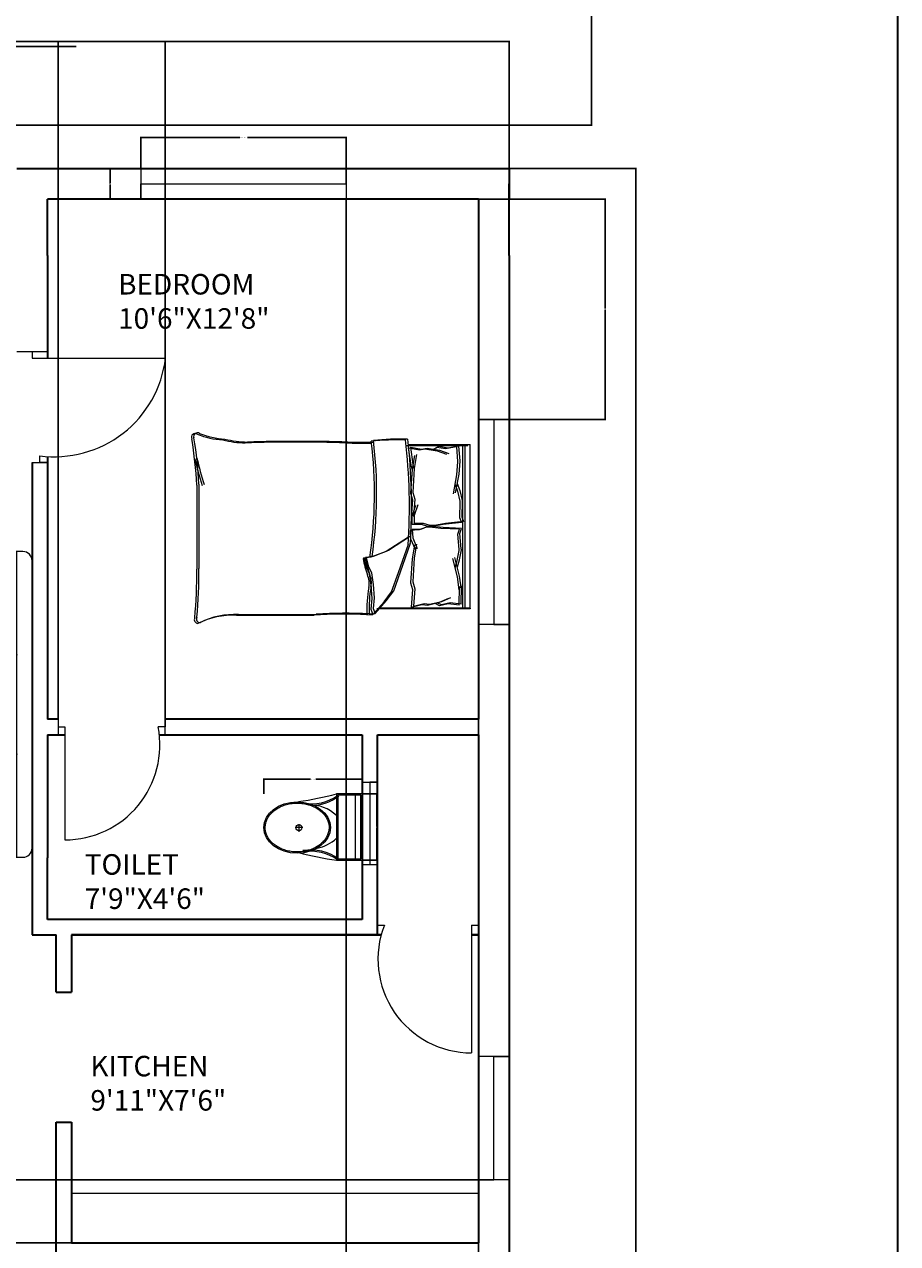
# Model space of a CAD drawing. Units: inches. Extents: x 1854 to 2495, y 1460 to 2772.
# Tile 11 of 12: x 2239 to 2495, y 1958 to 2314. Entities that reach past the tile are written whole.
import ezdxf

# ---------------------------------------------------------------- set-up
doc = ezdxf.new("R2010")
doc.units = ezdxf.units.IN
for name, color, linetype, lineweight in [('A-ANNO-DIMS', 2, 'Continuous', 18), ('A-ANNO-TEXT', 7, 'Continuous', 25), ('A-ANNO-TTLB', 7, 'Continuous', 35), ('A-AREA-IDEN', 7, 'Continuous', 18), ('A-DOOR', 3, 'Continuous', 18), ('A-FLOR-CASE', 8, 'Continuous', 18), ('A-FLOR-FIXT', 9, 'Continuous', 18), ('A-FURN', 8, 'Continuous', 13), ('A-GLAZ', 4, 'Continuous', 18), ('A-WALL', 7, 'Continuous', 35)]:
    doc.layers.add(name, color=color, linetype=linetype, lineweight=lineweight)
doc.styles.get("Standard").update_dxf_attribs({"font": 'arial.ttf'})
doc.dimstyles.get("Standard").update_dxf_attribs({"dimtxt": 0.18, "dimasz": 0.18, "dimexe": 0.18, "dimexo": 0.0625, "dimgap": 0.09, "dimtad": 0, "dimtih": 1, "dimtoh": 1, "dimdec": 4, "dimzin": 0, "dimdsep": 46, "dimtxsty": 'Standard', "dimcen": 0.09, "dimadec": 0, "dimazin": 0, "dimtfac": 1, "dimtdec": 4, "dimtofl": 0, "dimtmove": 0, "dimatfit": 3, "dimfxl": 1, "dimtolj": 1, "dimtzin": 0, "dimarcsym": 0})

# ---------------------------------------------------------------- blocks, each defined once
blk = doc.blocks.new('A$C31115884')
for p, q in [((283.1, 497.7), (223.4, 497.7)), ((257.5, 466.4), (257.5, 523.2)), ((0, 200), (0, 0)), ((520, 200), (0, 200)), ((520, 0), (520, 200)), ((10, 190), (10, 10)), ((510, 190), (10, 190)), ((510, 10), (510, 190)), ((510, 54.5), (0, 54.5)), ((10, 10), (510, 10)), ((0, 0), (520, 0))]:
    blk.add_line(p, q)
blk.add_circle((255.6, 496.4), 23.6)
for centre, radius, start, end in [((2777.7, -204.6), 2807, 165.4549, 171.71327), ((3237, 905), 2807, 188.28673, 194.5451), ((-294.5, 403.3), 364.7, 324.20913, 9.34987), ((-294.5, 403.3), 374.7, 324.20913, 9.34987), ((139.5, 406.2), 293.5, 315.84364, 2.65635), ((805.8, 403.3), 374.7, 179.20365, 215.79087), ((805.8, 403.3), 364.7, 170.65013, 215.79087), ((383.6, 406.2), 293.5, 190.27735, 224.15636)]:
    blk.add_arc(centre, radius, start, end)
blk.add_ellipse((256.2, 509.9), major_axis=(0, -260.7), ratio=0.772727)
blk.add_open_spline([(256.2, 259.2), (263.1, 259.2), (270, 259.7), (287.8, 262.3), (298.7, 265.1), (319.9, 273.1), (330.2, 278.4), (350.1, 291.1), (359.7, 298.7), (377.7, 315.9), (386.2, 325.5), (401.7, 346.6), (408.8, 358.1), (421.3, 382.5), (426.8, 395.5), (435.9, 422.4), (439.5, 436.4), (444.8, 465.1), (446.5, 479.7), (447.9, 509.2), (447.6, 524), (445, 553.3), (442.7, 567.8), (436.3, 596), (432.1, 609.7), (421.9, 636), (416, 648.6), (402.5, 672.1), (395, 683), (378.6, 703), (369.8, 712.1), (351.1, 728), (341.3, 734.8), (320.9, 746.2), (310.4, 750.7), (288.9, 757.3), (278, 759.4), (256, 761), (245, 760.6), (223.1, 757.2), (212.3, 754.3), (191.1, 746.1), (180.8, 740.7), (160.9, 727.8), (151.4, 720.1), (133.5, 702.7), (125.1, 693), (109.6, 671.7), (102.6, 660.2), (90.2, 635.7), (84.9, 622.7), (76, 595.6), (72.4, 581.6), (67.2, 552.9), (65.6, 538.2), (64.4, 508.8), (64.8, 494), (67.5, 464.7), (69.9, 450.2), (76.6, 422), (80.8, 408.3), (91.1, 382.2), (97.2, 369.7), (110.8, 346.3), (118.4, 335.4), (134.8, 315.6), (143.7, 306.7), (162.4, 290.9), (172.3, 284.2), (192.8, 273), (203.3, 268.6), (224.8, 262.2), (235.8, 260.2), (249.9, 259.3), (253, 259.2), (256.2, 259.2)], degree=3, knots=[0, 0, 0, 0, 0.110105, 0.110105, 0.285049, 0.285049, 0.459994, 0.459994, 0.634938, 0.634938, 0.809882, 0.809882, 0.984827, 0.984827, 1.159771, 1.159771, 1.334715, 1.334715, 1.50966, 1.50966, 1.684604, 1.684604, 1.859549, 1.859549, 2.034493, 2.034493, 2.209437, 2.209437, 2.384382, 2.384382, 2.559326, 2.559326, 2.73427, 2.73427, 2.909215, 2.909215, 3.084159, 3.084159, 3.259103, 3.259103, 3.434048, 3.434048, 3.608992, 3.608992, 3.783936, 3.783936, 3.958881, 3.958881, 4.133825, 4.133825, 4.30877, 4.30877, 4.483714, 4.483714, 4.658658, 4.658658, 4.833603, 4.833603, 5.008547, 5.008547, 5.183491, 5.183491, 5.358436, 5.358436, 5.53338, 5.53338, 5.708324, 5.708324, 5.883269, 5.883269, 6.058213, 6.058213, 6.233158, 6.233158, 6.283185, 6.283185, 6.283185, 6.283185])
blk = doc.blocks.new('BED-DOUBLE')
for p, q in [((0, 51.27), (0, 51.49)), ((0, 51.49), (0.64, 51.49)), ((0, 51.27), (26.61, 51.27)), ((0, 51.27), (26.61, 51.27)), ((0, 51.27), (0, 3.48)), ((0.64, 51.49), (27.25, 51.49)), ((0.64, 51.49), (27.25, 51.49)), ((1.53, 3.48), (1.53, 51.27)), ((1.53, 3.48), (1.53, 51.27)), ((2.17, 3.7), (2.17, 51.49)), ((2.17, 3.7), (2.17, 51.49)), ((2.56, 50.11), (2.46, 44.71)), ((2.56, 50.11), (2.46, 44.71)), ((2.56, 50.11), (5.77, 49.73)), ((2.56, 50.11), (5.77, 49.73)), ((3.2, 50.34), (3.1, 44.94)), ((3.2, 50.34), (3.1, 44.94)), ((3.2, 50.34), (6.41, 49.96)), ((3.2, 50.34), (6.41, 49.96)), ((5.77, 49.73), (8.34, 50.33)), ((5.77, 49.73), (8.34, 50.33)), ((6.41, 49.96), (8.98, 50.56)), ((6.41, 49.96), (8.98, 50.56)), ((11.83, 50.11), (8.26, 49.31)), ((11.83, 50.11), (8.26, 49.31)), ((8.34, 50.33), (9.38, 49.81)), ((8.34, 50.33), (9.38, 49.81)), ((12.47, 50.34), (8.9, 49.54)), ((12.47, 50.34), (8.9, 49.54)), ((8.98, 50.56), (10.02, 50.04)), ((8.98, 50.56), (10.02, 50.04)), ((13.43, 49.92), (11.83, 50.11)), ((13.43, 49.92), (11.83, 50.11)), ((14.07, 50.15), (12.47, 50.34)), ((14.07, 50.15), (12.47, 50.34)), ((16.57, 50.7), (13.43, 49.92)), ((16.57, 50.7), (13.43, 49.92)), ((17.21, 50.93), (14.07, 50.15)), ((17.21, 50.93), (14.07, 50.15)), ((16.17, 45.57), (16.57, 50.7)), ((16.17, 45.57), (16.57, 50.7)), ((16.81, 45.8), (17.21, 50.93)), ((16.81, 45.79), (17.21, 50.93)), ((27.75, 52.87), (24.5, 49.16)), ((27.75, 52.87), (24.5, 49.16)), ((28.39, 53.1), (25.14, 49.39)), ((28.39, 53.1), (25.14, 49.39)), ((29.49, 52.95), (27.75, 52.87, 3.87)), ((29.49, 52.95), (27.75, 52.87, 3.87)), ((28.37, 51.33), (27.75, 52.87)), ((28.37, 51.33), (27.75, 52.87)), ((28.06, 48.23), (28.37, 51.33)), ((28.06, 48.23), (28.37, 51.33)), ((30.13, 53.18), (28.39, 53.1, 3.87)), ((30.13, 53.18), (28.39, 53.1, 3.87)), ((29, 51.56), (28.39, 53.1)), ((29, 51.56), (28.39, 53.1)), ((28.7, 48.46), (29, 51.56)), ((28.7, 48.46), (29, 51.56)), ((8.26, 49.31), (5.58, 48.13)), ((8.26, 49.31), (5.58, 48.13)), ((8.9, 49.54), (6.22, 48.36)), ((8.9, 49.54), (6.22, 48.36)), ((22.97, 46.45), (20.96, 40.87)), ((22.97, 46.45), (20.96, 40.87)), ((24.5, 49.16), (22.33, 46.22)), ((24.5, 49.16), (22.33, 46.22)), ((25.14, 49.39), (22.97, 46.45)), ((25.14, 49.39), (22.97, 46.45)), ((28.37, 44.36), (28.06, 48.23)), ((28.37, 44.36), (28.06, 48.23)), ((29, 44.59), (28.7, 48.46)), ((29, 44.59), (28.7, 48.46)), ((2.46, 44.71), (2.54, 45.71)), ((2.46, 44.71), (2.54, 45.71)), ((2.54, 45.71), (3.07, 41.91)), ((2.54, 45.71), (3.07, 41.91)), ((3.1, 44.94), (3.18, 45.94)), ((3.1, 44.94), (3.18, 45.94)), ((3.18, 45.94), (3.71, 42.14)), ((3.18, 45.94), (3.71, 42.14)), ((16.73, 43.61), (16.17, 45.57)), ((16.73, 43.61), (16.17, 45.57)), ((16.3, 36.6), (16.73, 43.61)), ((16.3, 36.6), (16.73, 43.61)), ((17.37, 43.83), (16.81, 45.8)), ((17.37, 43.83), (16.81, 45.79)), ((16.93, 36.82), (17.37, 43.83)), ((16.93, 36.82), (17.37, 43.83)), ((22.33, 46.22), (20.32, 40.64)), ((22.33, 46.22), (20.32, 40.64)), ((28.83, 40.95), (28.37, 44.36)), ((28.83, 40.95), (28.37, 44.36)), ((29.47, 41.18), (29, 44.59)), ((29.47, 41.18), (29, 44.59)), ((3.07, 41.91), (4.42, 36.5)), ((3.07, 41.91), (4.42, 36.5)), ((3.67, 39.2), (3.08, 37.14)), ((3.67, 39.2), (3.08, 37.14)), ((3.71, 42.14), (5.06, 36.72)), ((3.71, 42.14), (5.06, 36.72)), ((4.31, 39.43), (3.72, 37.36)), ((4.31, 39.43), (3.72, 37.36)), ((20.32, 40.64), (17.38, 32.31)), ((20.32, 40.64), (17.38, 32.31)), ((20.96, 40.87), (18.02, 32.53)), ((20.96, 40.87), (18.02, 32.53)), ((29.76, 38.94), (28.83, 40.95)), ((29.76, 38.94), (28.83, 40.95)), ((30.4, 39.17), (29.47, 41.18)), ((30.4, 39.17), (29.47, 41.18)), ((79.25, 15.06), (79.25, 39.68)), ((79.25, 15.06), (79.25, 39.68)), ((79.88, 15.29), (79.88, 39.91)), ((79.88, 15.29), (79.88, 39.91)), ((3.08, 37.14), (2.54, 34.2)), ((3.08, 37.14), (2.54, 34.2)), ((3.72, 37.36), (3.18, 34.43)), ((3.72, 37.36), (3.18, 34.43)), ((15.63, 32.56), (16.3, 36.6)), ((15.63, 32.56), (16.3, 36.6)), ((16.27, 32.79), (16.93, 36.82)), ((16.27, 32.79), (16.93, 36.82)), ((23.88, 34.45), (28.37, 36.15)), ((23.88, 34.45), (28.37, 36.15)), ((24.52, 34.68), (29, 36.38)), ((24.52, 34.68), (29, 36.38)), ((28.37, 36.15), (30.38, 36.46)), ((28.37, 36.15), (30.38, 36.46)), ((29, 36.38), (31.02, 36.69)), ((29, 36.38), (31.02, 36.69)), ((30.38, 36.46), (29.76, 38.94)), ((30.38, 36.46), (29.76, 38.94)), ((31.02, 36.69), (30.4, 39.17)), ((31.02, 36.69), (30.4, 39.17)), ((2.54, 34.2), (2.56, 33.88)), ((2.54, 34.2), (2.56, 33.88)), ((2.56, 33.88), (2.98, 29.46)), ((2.56, 33.88), (2.98, 29.46)), ((3.18, 34.43), (3.2, 34.11)), ((3.18, 34.43), (3.2, 34.11)), ((3.2, 34.11), (3.62, 29.68)), ((3.2, 34.11), (3.62, 29.68)), ((16.74, 30.75), (15.45, 33.82)), ((16.74, 30.75), (15.45, 33.82)), ((17.38, 30.98), (16.09, 34.05)), ((17.38, 30.98), (16.09, 34.05)), ((17.38, 30.26), (23.88, 34.45)), ((17.38, 30.26), (23.88, 34.45)), ((18.02, 30.49), (24.52, 34.68)), ((18.02, 30.49), (24.52, 34.68)), ((2.98, 29.46), (2.49, 27.98)), ((2.98, 29.46), (2.49, 27.98)), ((3.62, 29.68), (3.13, 28.21)), ((3.62, 29.68), (3.13, 28.21)), ((14.86, 28.36), (17.53, 28.53)), ((14.86, 28.36), (17.53, 28.53)), ((16.89, 28.3), (16.74, 30.75)), ((16.89, 28.3), (16.74, 30.75)), ((17.53, 28.53), (17.38, 30.98)), ((17.53, 28.53), (17.38, 30.98)), ((1.87, 25.98), (7.22, 26.56)), ((1.87, 25.98), (7.22, 26.56)), ((2.45, 24.54), (1.87, 25.98)), ((2.45, 24.54), (1.87, 25.98)), ((2.49, 27.98), (7.87, 27.73)), ((2.49, 27.98), (7.87, 27.73)), ((2.51, 26.21), (7.86, 26.79)), ((2.51, 26.21), (7.86, 26.79)), ((3.09, 24.77), (2.51, 26.21)), ((3.09, 24.77), (2.51, 26.21)), ((3.13, 28.21), (8.51, 27.96)), ((3.13, 28.21), (8.51, 27.96)), ((7.22, 26.56), (10.4, 27.14)), ((7.22, 26.56), (10.4, 27.14)), ((7.86, 26.79), (11.04, 27.37)), ((7.86, 26.79), (11.04, 27.37)), ((7.87, 27.73), (11.08, 27.36)), ((7.87, 27.73), (11.08, 27.35)), ((8.51, 27.96), (11.72, 27.58)), ((8.51, 27.96), (11.72, 27.58)), ((10.4, 27.14), (11.7, 27.14)), ((10.4, 27.14), (11.7, 27.14)), ((11.04, 27.37), (12.34, 27.37)), ((11.04, 27.37), (12.34, 27.37)), ((11.08, 27.36), (12.38, 27.44)), ((11.08, 27.35), (12.38, 27.44)), ((11.7, 27.14), (13.58, 26.56)), ((11.7, 27.14), (13.58, 26.56)), ((11.72, 27.58), (13.02, 27.66)), ((11.72, 27.58), (13.02, 27.66)), ((12.34, 27.37), (14.22, 26.79)), ((12.34, 27.37), (14.22, 26.79)), ((12.38, 27.44), (14.22, 28.13)), ((12.38, 27.44), (14.22, 28.13)), ((13.02, 27.66), (14.86, 28.36)), ((13.02, 27.66), (14.86, 28.36)), ((13.58, 26.56), (16.26, 26.56)), ((13.58, 26.56), (16.26, 26.56)), ((14.22, 28.13), (16.89, 28.3)), ((14.22, 28.13), (16.89, 28.3)), ((14.22, 26.79), (16.9, 26.79)), ((14.22, 26.79), (16.9, 26.79)), ((16.26, 26.56), (16.26, 24.1)), ((16.26, 26.56), (16.26, 24.1)), ((16.9, 26.79), (16.9, 24.33)), ((16.9, 26.79), (16.9, 24.33)), ((2.3, 20.09), (2.45, 24.54)), ((2.3, 20.09), (2.45, 24.54)), ((2.94, 20.32), (3.09, 24.77)), ((2.94, 20.32), (3.09, 24.77)), ((16.26, 24.1), (15.17, 20.96)), ((16.26, 24.1), (15.17, 20.96)), ((16.9, 24.33), (15.81, 21.19)), ((16.9, 24.33), (15.81, 21.19)), ((16.17, 19.38), (16.57, 24.52)), ((16.17, 19.38), (16.57, 24.52)), ((16.81, 19.61), (17.21, 24.74)), ((16.81, 19.61), (17.21, 24.74)), ((2.3, 19.77), (2.3, 20.09)), ((2.3, 19.77), (2.3, 20.09)), ((3.03, 16.88), (2.3, 19.77)), ((3.03, 16.88), (2.3, 19.77)), ((2.94, 20), (2.94, 20.32)), ((2.94, 20), (2.94, 20.32)), ((3.67, 17.11), (2.94, 20)), ((3.67, 17.11), (2.94, 20)), ((3.96, 12.34), (4.97, 17.83)), ((3.96, 12.34), (4.97, 17.83)), ((16.73, 17.42), (16.17, 19.38)), ((16.73, 17.42), (16.17, 19.38)), ((17.37, 17.65), (16.81, 19.61)), ((17.37, 17.65), (16.81, 19.61)), ((3.75, 14.86), (3.03, 16.88)), ((3.75, 14.85), (3.03, 16.88)), ((3.32, 12.11), (4.33, 17.6)), ((3.32, 12.11), (4.33, 17.6)), ((4.39, 15.08), (3.67, 17.11)), ((4.39, 15.08), (3.67, 17.11)), ((16.3, 10.41), (16.73, 17.42)), ((16.3, 10.41), (16.73, 17.42)), ((16.93, 10.64), (17.37, 17.65)), ((16.93, 10.64), (17.37, 17.65)), ((3.03, 8.29), (3.32, 12.11)), ((3.03, 8.28), (3.32, 12.11)), ((3.67, 8.51), (3.96, 12.34)), ((3.67, 8.51), (3.96, 12.34)), ((3.01, 8.18), (3.03, 8.29)), ((3.01, 8.18), (3.03, 8.28)), ((3.34, 3.9), (3.01, 8.18)), ((3.34, 3.9), (3.01, 8.18)), ((3.65, 8.41), (3.67, 8.51)), ((3.65, 8.41), (3.67, 8.51)), ((3.98, 4.13), (3.65, 8.41)), ((3.98, 4.13), (3.65, 8.41)), ((15.63, 6.38), (16.3, 10.41)), ((15.63, 6.38), (16.3, 10.41)), ((16.27, 6.61), (16.93, 10.64)), ((16.27, 6.61), (16.93, 10.64)), ((16.3, 10.41), (16.62, 9.28)), ((16.3, 10.41), (16.62, 9.28)), ((16.62, 9.28), (17.34, 4.18)), ((16.62, 9.28), (17.34, 4.18)), ((16.93, 10.64), (17.26, 9.51)), ((16.93, 10.64), (17.26, 9.51)), ((17.26, 9.51), (17.98, 4.41)), ((17.26, 9.51), (17.98, 4.41)), ((18.75, 3.7), (0.64, 3.7)), ((18.75, 3.7), (0.64, 3.7)), ((3.32, 3.89), (6.5, 4.47)), ((3.32, 3.89), (6.5, 4.47)), ((3.96, 4.12), (7.14, 4.7)), ((3.96, 4.12), (7.14, 4.7)), ((8.96, 5.05), (6.21, 6.06)), ((8.96, 5.05), (6.21, 6.06)), ((6.5, 4.47), (9.1, 4.04)), ((6.5, 4.47), (9.1, 4.04)), ((9.59, 5.28), (6.85, 6.29)), ((9.59, 5.28), (6.85, 6.29)), ((7.14, 4.7), (9.74, 4.27)), ((7.14, 4.7), (9.74, 4.27)), ((12.57, 4.47), (8.96, 5.05)), ((12.57, 4.47), (8.96, 5.05)), ((9.1, 4.04), (10.11, 4.62)), ((9.1, 4.04), (10.11, 4.62)), ((13.21, 4.7), (9.59, 5.28)), ((13.21, 4.7), (9.59, 5.28)), ((9.74, 4.27), (10.75, 4.85)), ((9.74, 4.27), (10.75, 4.85)), ((14.16, 4.76), (12.57, 4.47)), ((14.16, 4.76), (12.57, 4.47)), ((14.8, 4.99), (13.21, 4.7)), ((14.8, 4.99), (13.21, 4.7)), ((17.34, 4.18), (14.16, 4.76)), ((17.34, 4.18), (14.16, 4.76)), ((17.98, 4.41), (14.8, 4.99)), ((17.98, 4.41), (14.8, 4.99)), ((18.11, 3.48), (0, 3.48)), ((18.11, 3.48), (0, 3.48))]:
    blk.add_line(p, q)
for centre, radius, start, end in [((68.67, 76.16), 23.07, 267.4714, 296.4681), ((68.67, 76.16), 23.07, 267.4714, 296.4681), ((69.31, 76.39), 23.07, 267.4714, 296.4681), ((69.31, 76.39), 23.07, 267.4714, 296.4681), ((78.87, 54.41), 1.1, 332.6588, 86.02), ((78.87, 54.41), 1.1, 332.6588, 86.02), ((212.28, 41.15), 133.04, 174.4998, 180.6351), ((212.28, 41.15), 133.04, 174.4998, 180.6351), ((79.51, 54.64), 1.1, 332.6588, 86.02), ((79.51, 54.64), 1.1, 332.6588, 86.02), ((212.92, 41.38), 133.04, 174.4998, 180.6351), ((212.92, 41.38), 133.04, 174.4998, 180.6351), ((-6.66, 51.33), 36.18, 349.8763, 2.5657), ((-6.66, 51.33), 36.18, 349.8763, 2.5657), ((36.32, 182.27), 129.5, 266.9791, 273.8365), ((36.32, 182.27), 129.5, 266.9791, 273.8365), ((-6.02, 51.56), 36.18, 349.8763, 2.5657), ((-6.02, 51.56), 36.18, 349.8763, 2.5657), ((36.95, 182.49), 129.5, 266.9791, 273.8365), ((36.95, 182.49), 129.5, 266.9791, 273.8365), ((67.82, -4508.74), 4561.86, 90.00217, 90.28689), ((67.82, -4508.74), 4561.86, 90.00217, 90.28689), ((68.46, -4508.51), 4561.86, 90.00217, 90.28689), ((68.46, -4508.52), 4561.86, 90.00217, 90.28689), ((35.07, 43.74), 6.22, 168.6608, 203.7384), ((35.07, 43.74), 6.22, 168.6608, 203.7384), ((35.71, 43.97), 6.22, 168.6608, 203.7384), ((35.71, 43.97), 6.22, 168.6608, 203.7384), ((1.48, 31.15), 29.65, 10.6617, 19.8806), ((1.48, 31.15), 29.65, 10.6617, 19.8806), ((2.12, 31.38), 29.65, 10.6617, 19.8806), ((2.12, 31.38), 29.65, 10.6617, 19.8806), ((156.32, 17.76), 129.02, 171.7845, 186.9006), ((156.32, 17.76), 129.02, 171.7845, 186.9006), ((156.96, 17.98), 129.02, 171.7845, 186.9006), ((156.96, 17.98), 129.02, 171.7845, 186.9006), ((30.44, 36.64), 0.185, 250.2464, 1.1377), ((30.44, 36.64), 0.185, 250.2464, 1.1377), ((31.08, 36.86), 0.185, 250.2464, 1.1377), ((31.08, 36.86), 0.185, 250.2464, 1.1377), ((182.05, 21.36), 164.97, 176.0865, 186.7821), ((182.05, 21.36), 164.97, 176.0865, 186.7821), ((182.69, 21.59), 164.97, 176.0865, 186.7821), ((182.69, 21.59), 164.97, 176.0865, 186.7821), ((-23.71, -17.22), 106.46, 13.3832, 17.7053), ((-23.71, -17.22), 106.46, 13.3832, 17.7053), ((-23.07, -16.99), 106.46, 13.3832, 17.7053), ((-23.07, -16.99), 106.46, 13.3832, 17.7053), ((200.84, 21.43), 121.76, 182.9958, 189.4091), ((200.84, 21.43), 121.76, 182.9958, 189.4091), ((201.48, 21.66), 121.76, 182.9958, 189.4091), ((201.48, 21.66), 121.76, 182.9958, 189.4091), ((20.1, 85.16), 83.31, 268.7218, 275.604), ((20.1, 85.16), 83.31, 268.7218, 275.604), ((20.74, 85.39), 83.31, 268.7218, 275.604), ((20.74, 85.39), 83.31, 268.7218, 275.604), ((31.17, -167.31), 170.11, 88.4762, 91.0082), ((31.17, -167.31), 170.11, 88.4762, 91.0082), ((31.81, -167.08), 170.11, 88.4762, 91.0082), ((31.81, -167.08), 170.11, 88.4762, 91.0082), ((50.61, 484.82), 482.31, 268.2277, 271.7185), ((50.61, 484.82), 482.31, 268.2277, 271.7185), ((51.25, 485.05), 482.31, 268.2277, 271.7185), ((51.25, 485.05), 482.31, 268.2277, 271.7185), ((64.52, -26.9), 29.63, 76.0648, 88.9113), ((64.52, -26.9), 29.63, 76.0648, 88.9113), ((65.15, -26.67), 29.63, 76.0648, 88.9113), ((65.15, -26.67), 29.63, 76.0648, 88.9113), ((70.28, -21.66), 23.56, 67.9751, 86.652), ((70.28, -21.66), 23.56, 67.9751, 86.652), ((70.92, -21.43), 23.56, 67.9751, 86.652), ((70.92, -21.43), 23.56, 67.9751, 86.652), ((79.72, 1.09), 1.09, 236.1736, 23.4781), ((79.72, 1.09), 1.09, 236.1736, 23.4781), ((80.36, 1.32), 1.09, 236.1736, 23.4781), ((80.36, 1.32), 1.09, 236.1736, 23.4781)]:
    blk.add_arc(centre, radius, start, end)
blk = doc.blocks.new('WINDOW-60IN')
for p, q in [((0, 9), (0, 0)), ((60, 4.5), (60, 9)), ((60, 9), (60, 0)), ((0, 0), (0, 4.5)), ((0, 4.5), (60, 4.5))]:
    blk.add_line(p, q)
blk = doc.blocks.new('WINDOW-36IN')
for p, q in [((0, 36), (9, 36)), ((9, 36), (4.5, 36)), ((4.5, 36), (4.5, 0)), ((4.5, 0), (0, 0)), ((0, 0), (9, 0))]:
    blk.add_line(p, q)
blk = doc.blocks.new('WINDOW-VENT-24IN-INTERIOR')
for p, q in [((0, 24), (4.5, 24)), ((2.25, 24), (2.25, 0)), ((0, 0), (4.5, 0))]:
    blk.add_line(p, q)
blk = doc.blocks.new('SOFA-3-SEAT')
for points in [[(2.23, 59.19), (21.22, 59.19, 0.414214), (23.45, 61.43), (23.45, 87.12, 0.414214), (21.22, 89.35), (2.23, 89.35, 0.414214), (0, 87.12), (0, 61.43, 0.414214)], [(2.23, 59.19), (21.22, 59.19, -0.414214), (23.45, 56.96), (23.45, 32.39, -0.414214), (21.22, 30.16), (2.23, 30.16, -0.414214), (0, 32.39), (0, 56.96, -0.414214)], [(2.23, 0), (21.22, 0, 0.414214), (23.45, 2.23), (23.45, 27.92, 0.414214), (21.22, 30.16), (2.23, 30.16, 0.414214), (0, 27.92), (0, 2.23, 0.414214)]]:
    blk.add_lwpolyline(points, format="xyb", close=True)
at = {"ltscale": 0.03}
blk.add_lwpolyline([(0, 28.35), (0, 1.79, 0.414214), (1.79, 0), (28.59, 0, 0.414214), (31.27, 2.68), (31.27, 86.67, 0.414214), (28.59, 89.35), (1.79, 89.35, 0.414214), (0, 87.56), (0, 61, 0.414214), (1.79, 59.22, -1), (1.79, 59.17, 0.414214), (0, 57.38), (0, 31.96, 0.414214), (1.79, 30.18, -1), (1.79, 30.13, 0.414214)], format="xyb", close=True, dxfattribs=at)
blk.add_lwpolyline([(26.8, 0), (26.8, 89.35)])
for centre, radius, start, end in [((58.64, 74.27), 35.22, 154.6538, 205.3462), ((56.4, 44.67), 32.97, 153.869, 206.131), ((59.01, 15.08), 35.56, 154.9106, 205.0894)]:
    blk.add_arc(centre, radius, start, end)
blk = doc.blocks.new('*D17')
at = {"layer": 'A-ANNO-DIMS', "color": 0, "lineweight": -2, "transparency": 16777216}
for p, q in [((2273.32, 2272.11), (2273.32, 2281.22)), ((2273.5, 2281.04), (2302.2, 2281.04)), ((2333.14, 2281.04), (2304.44, 2281.04)), ((2333.32, 2272.11), (2333.32, 2281.22))]:
    blk.add_line(p, q, dxfattribs=at)
at = {"layer": 'A-ANNO-DIMS', "color": 0, "transparency": 16777216}
for points in [[(2273.5, 2281.07), (2273.5, 2281.01), (2273.32, 2281.04)], [(2333.14, 2281.07), (2333.14, 2281.01), (2333.32, 2281.04)]]:
    blk.add_solid(points, dxfattribs=at)
at = {"layer": 'Defpoints', "color": 0, "transparency": 16777216}
for p in [(2333.32, 2281.04), (2273.32, 2272.04), (2333.32, 2272.04)]:
    blk.add_point(p, dxfattribs=at)
at = {"layer": 'A-ANNO-DIMS', "color": 0, "transparency": 16777216, "insert": (2303.32, 2281.04), "char_height": 0.18, "attachment_point": 5}
blk.add_mtext('\\A1;WINDOW 60 TYP.', dxfattribs=at)
blk = doc.blocks.new('*D18')
at = {"layer": 'A-ANNO-DIMS', "color": 0, "lineweight": -2, "transparency": 16777216}
for p, q in [((2273.26, 2272.04), (2264.14, 2272.04)), ((2264.32, 2271.86), (2264.32, 2267.73)), ((2264.32, 2263.22), (2264.32, 2267.36)), ((2273.26, 2263.04), (2264.14, 2263.04))]:
    blk.add_line(p, q, dxfattribs=at)
at = {"layer": 'A-ANNO-DIMS', "color": 0, "transparency": 16777216}
for points in [[(2264.29, 2271.86), (2264.35, 2271.86), (2264.32, 2272.04)], [(2264.29, 2263.22), (2264.35, 2263.22), (2264.32, 2263.04)]]:
    blk.add_solid(points, dxfattribs=at)
at = {"layer": 'Defpoints', "color": 0, "transparency": 16777216}
for p in [(2264.32, 2272.04), (2273.32, 2272.04), (2273.32, 2263.04)]:
    blk.add_point(p, dxfattribs=at)
at = {"layer": 'A-ANNO-DIMS', "color": 0, "transparency": 16777216, "insert": (2264.32, 2267.54), "char_height": 0.18, "attachment_point": 5}
blk.add_mtext('\\A1;9 TYP.', dxfattribs=at)
blk = doc.blocks.new('*D19')
at = {"layer": 'A-ANNO-DIMS', "color": 0, "lineweight": -2, "transparency": 16777216}
for p, q in [((2309.26, 2089.3), (2309.26, 2093.72)), ((2309.44, 2093.54), (2322.85, 2093.54)), ((2337.8, 2093.54), (2324.4, 2093.54)), ((2337.98, 2089.3), (2337.98, 2093.72))]:
    blk.add_line(p, q, dxfattribs=at)
at = {"layer": 'A-ANNO-DIMS', "color": 0, "transparency": 16777216}
for points in [[(2309.44, 2093.57), (2309.44, 2093.51), (2309.26, 2093.54)], [(2337.8, 2093.57), (2337.8, 2093.51), (2337.98, 2093.54)]]:
    blk.add_solid(points, dxfattribs=at)
at = {"layer": 'Defpoints', "color": 0, "transparency": 16777216}
for p in [(2309.26, 2093.54), (2309.26, 2089.24), (2337.98, 2089.24)]:
    blk.add_point(p, dxfattribs=at)
at = {"layer": 'A-ANNO-DIMS', "color": 0, "transparency": 16777216, "insert": (2323.62, 2093.54), "char_height": 0.18, "attachment_point": 5}
blk.add_mtext('\\A1;WC 29 TYP.', dxfattribs=at)
blk = doc.blocks.new('*D20')
at = {"layer": 'A-ANNO-DIMS', "color": 0, "lineweight": -2, "transparency": 16777216}
for p, q in [((2338.04, 2089.24), (2342.47, 2089.24)), ((2342.29, 2089.06), (2342.29, 2079.73)), ((2342.29, 2070.03), (2342.29, 2079.36)), ((2338.04, 2069.85), (2342.47, 2069.85))]:
    blk.add_line(p, q, dxfattribs=at)
at = {"layer": 'A-ANNO-DIMS', "color": 0, "transparency": 16777216}
for points in [[(2342.26, 2089.06), (2342.32, 2089.06), (2342.29, 2089.24)], [(2342.26, 2070.03), (2342.32, 2070.03), (2342.29, 2069.85)]]:
    blk.add_solid(points, dxfattribs=at)
at = {"layer": 'Defpoints', "color": 0, "transparency": 16777216}
for p in [(2337.98, 2089.24), (2342.29, 2089.24), (2337.98, 2069.85)]:
    blk.add_point(p, dxfattribs=at)
at = {"layer": 'A-ANNO-DIMS', "color": 0, "transparency": 16777216, "insert": (2342.29, 2079.54), "char_height": 0.18, "attachment_point": 5}
blk.add_mtext('\\A1;19 TYP.', dxfattribs=at)
blk = doc.blocks.new('*D49')
at = {"layer": 'A-ANNO-DIMS', "color": 0, "lineweight": -2, "transparency": 16777216}
for p, q in [((1977.98, 2246.51), (1977.98, 2309.27)), ((1978.16, 2309.09), (2179.19, 2309.09)), ((2380.8, 2309.09), (2179.77, 2309.09)), ((2380.98, 2272.11), (2380.98, 2309.27))]:
    blk.add_line(p, q, dxfattribs=at)
at = {"layer": 'A-ANNO-DIMS', "color": 0, "transparency": 16777216}
for points in [[(1978.16, 2309.12), (1978.16, 2309.06), (1977.98, 2309.09)], [(2380.8, 2309.12), (2380.8, 2309.06), (2380.98, 2309.09)]]:
    blk.add_solid(points, dxfattribs=at)
at = {"layer": 'Defpoints', "color": 0, "transparency": 16777216}
for p in [(2380.98, 2309.09), (2380.98, 2272.04), (1977.98, 2246.45)]:
    blk.add_point(p, dxfattribs=at)
at = {"layer": 'A-ANNO-DIMS', "color": 0, "transparency": 16777216, "insert": (2179.48, 2309.09), "char_height": 0.18, "attachment_point": 5}
blk.add_mtext('\\A1;403', dxfattribs=at)
blk = doc.blocks.new('*D50')
at = {"layer": 'A-ANNO-DIMS', "color": 0, "lineweight": -2, "transparency": 16777216}
for p, q in [((2381.04, 2272.04), (2418.21, 2272.04)), ((2418.03, 2271.86), (2418.03, 1933.48)), ((2418.03, 1594.72), (2418.03, 1933.11)), ((2119.04, 1594.54), (2418.21, 1594.54))]:
    blk.add_line(p, q, dxfattribs=at)
at = {"layer": 'A-ANNO-DIMS', "color": 0, "transparency": 16777216}
for points in [[(2418, 2271.86), (2418.06, 2271.86), (2418.03, 2272.04)], [(2418, 1594.72), (2418.06, 1594.72), (2418.03, 1594.54)]]:
    blk.add_solid(points, dxfattribs=at)
at = {"layer": 'Defpoints', "color": 0, "transparency": 16777216}
for p in [(2380.98, 2272.04), (2418.03, 2272.04), (2118.98, 1594.54)]:
    blk.add_point(p, dxfattribs=at)
at = {"layer": 'A-ANNO-DIMS', "color": 0, "transparency": 16777216, "insert": (2418.03, 1933.29), "char_height": 0.18, "attachment_point": 5}
blk.add_mtext('\\A1;677.5', dxfattribs=at)
blk = doc.blocks.new('*D64')
at = {"layer": 'A-ANNO-DIMS', "color": 0, "lineweight": -2, "transparency": 16777216}
for p, q in [((2333.32, 2262.98), (2333.32, 1503.44)), ((2371.98, 2262.98), (2371.98, 1503.44)), ((2333.5, 1503.62), (2352.26, 1503.62)), ((2371.8, 1503.62), (2353.05, 1503.62))]:
    blk.add_line(p, q, dxfattribs=at)
at = {"layer": 'A-ANNO-DIMS', "color": 0, "transparency": 16777216}
for points in [[(2333.5, 1503.65), (2333.5, 1503.59), (2333.32, 1503.62)], [(2371.8, 1503.65), (2371.8, 1503.59), (2371.98, 1503.62)]]:
    blk.add_solid(points, dxfattribs=at)
at = {"layer": 'Defpoints', "color": 0, "transparency": 16777216}
for p in [(2333.32, 2263.04), (2371.98, 2263.04), (2371.98, 1503.62)]:
    blk.add_point(p, dxfattribs=at)
at = {"layer": 'A-ANNO-DIMS', "color": 0, "transparency": 16777216, "insert": (2352.65, 1503.62), "char_height": 0.18, "attachment_point": 5}
blk.add_mtext('\\A1;38.66', dxfattribs=at)
blk = doc.blocks.new('*D65')
at = {"layer": 'A-ANNO-DIMS', "color": 0, "lineweight": -2, "transparency": 16777216}
for p, q in [((2372.04, 2263.04), (2409.21, 2263.04)), ((2409.03, 2262.86), (2409.03, 2231.05)), ((2409.03, 2198.88), (2409.03, 2230.69)), ((2372.04, 2198.7), (2409.21, 2198.7))]:
    blk.add_line(p, q, dxfattribs=at)
at = {"layer": 'A-ANNO-DIMS', "color": 0, "transparency": 16777216}
for points in [[(2409, 2262.86), (2409.06, 2262.86), (2409.03, 2263.04)], [(2409, 2198.88), (2409.06, 2198.88), (2409.03, 2198.7)]]:
    blk.add_solid(points, dxfattribs=at)
at = {"layer": 'Defpoints', "color": 0, "transparency": 16777216}
for p in [(2371.98, 2263.04), (2371.98, 2198.7), (2409.03, 2198.7)]:
    blk.add_point(p, dxfattribs=at)
at = {"layer": 'A-ANNO-DIMS', "color": 0, "transparency": 16777216, "insert": (2409.03, 2230.87), "char_height": 0.18, "attachment_point": 5}
blk.add_mtext('\\A1;64.35', dxfattribs=at)
blk = doc.blocks.new('*D68')
at = {"layer": 'A-ANNO-DIMS', "color": 0, "lineweight": -2, "transparency": 16777216}
for p, q in [((2371.92, 1976.49), (1940.75, 1976.49)), ((1940.93, 1976.31), (1940.93, 1967.45)), ((1940.93, 1958.22), (1940.93, 1967.08)), ((2371.92, 1958.04), (1940.75, 1958.04))]:
    blk.add_line(p, q, dxfattribs=at)
at = {"layer": 'A-ANNO-DIMS', "color": 0, "transparency": 16777216}
for points in [[(1940.9, 1976.31), (1940.96, 1976.31), (1940.93, 1976.49)], [(1940.9, 1958.22), (1940.96, 1958.22), (1940.93, 1958.04)]]:
    blk.add_solid(points, dxfattribs=at)
at = {"layer": 'Defpoints', "color": 0, "transparency": 16777216}
for p in [(2371.98, 1976.49), (1940.93, 1958.04), (2371.98, 1958.04)]:
    blk.add_point(p, dxfattribs=at)
at = {"layer": 'A-ANNO-DIMS', "color": 0, "transparency": 16777216, "insert": (1940.93, 1967.27), "char_height": 0.18, "attachment_point": 5}
blk.add_mtext('\\A1;18.442', dxfattribs=at)
blk = doc.blocks.new('*D72')
at = {"layer": 'A-ANNO-DIMS', "color": 0, "lineweight": -2, "transparency": 16777216}
for p, q in [((2249.09, 2111.11), (2249.09, 2309.27)), ((2249.27, 2309.09), (2264.33, 2309.09)), ((2280.17, 2309.09), (2265.12, 2309.09)), ((2280.35, 2111.11), (2280.35, 2309.27))]:
    blk.add_line(p, q, dxfattribs=at)
at = {"layer": 'A-ANNO-DIMS', "color": 0, "transparency": 16777216}
for points in [[(2249.27, 2309.12), (2249.27, 2309.06), (2249.09, 2309.09)], [(2280.17, 2309.12), (2280.17, 2309.06), (2280.35, 2309.09)]]:
    blk.add_solid(points, dxfattribs=at)
at = {"layer": 'Defpoints', "color": 0, "transparency": 16777216}
for p in [(2280.35, 2309.09), (2249.09, 2111.04), (2280.35, 2111.04)]:
    blk.add_point(p, dxfattribs=at)
at = {"layer": 'A-ANNO-DIMS', "color": 0, "transparency": 16777216, "insert": (2264.72, 2309.09), "char_height": 0.18, "attachment_point": 5}
blk.add_mtext('\\A1;31.26', dxfattribs=at)
blk = doc.blocks.new('*D74')
at = {"layer": 'A-ANNO-DIMS', "color": 0, "lineweight": -2, "transparency": 16777216}
for p, q in [((1953.98, 2372.03), (1953.98, 2284.46)), ((2404.98, 2372.03), (2404.98, 2284.46)), ((1954.16, 2284.64), (2179.21, 2284.64)), ((2404.8, 2284.64), (2179.76, 2284.64))]:
    blk.add_line(p, q, dxfattribs=at)
at = {"layer": 'A-ANNO-DIMS', "color": 0, "transparency": 16777216}
for points in [[(1954.16, 2284.67), (1954.16, 2284.61), (1953.98, 2284.64)], [(2404.8, 2284.67), (2404.8, 2284.61), (2404.98, 2284.64)]]:
    blk.add_solid(points, dxfattribs=at)
at = {"layer": 'Defpoints', "color": 0, "transparency": 16777216}
for p in [(1953.98, 2372.09), (2404.98, 2372.09), (2404.98, 2284.64)]:
    blk.add_point(p, dxfattribs=at)
at = {"layer": 'A-ANNO-DIMS', "color": 0, "transparency": 16777216, "insert": (2179.48, 2284.64), "char_height": 0.18, "attachment_point": 5}
blk.add_mtext('\\A1;451', dxfattribs=at)

msp = doc.modelspace()

# ---------------------------------------------------------------- linework, layer by layer
at = {"layer": 'A-ANNO-TEXT'}
msp.add_line((2103.8101, 2307.6905), (2254.3702, 2307.6905), dxfattribs=at)
at = {"layer": 'A-ANNO-TTLB'}
msp.add_lwpolyline([(1854.1764, 2772.4852), (2494.521, 2772.4852), (2494.521, 1460.4076), (1854.1764, 1460.4076)], close=True, dxfattribs=at)
at = {"layer": 'A-DOOR'}
for p, q in [((2236.9824, 2218.5567), (2245.9824, 2218.5567)), ((2241.4824, 2218.5567), (2241.4824, 2216.5567)), ((2241.4824, 2218.5567), (2241.4824, 2216.5567)), ((2241.4824, 2216.5567), (2277.4824, 2216.5567)), ((2277.4824, 2216.5567), (2280.4824, 2216.5567)), ((2243.7324, 2186.0549), (2243.7324, 2188.0549)), ((2241.4824, 2186.0549), (2245.9824, 2186.0549)), ((2245.9824, 2186.0549), (2243.7324, 2186.0549)), ((2245.9824, 2186.0549), (2245.9824, 2186.0549)), ((2249.0932, 2111.0449), (2249.0932, 2106.5449)), ((2280.3522, 2106.5449), (2280.3522, 2111.0449)), ((2280.3522, 2111.0449), (2280.3522, 2108.7949)), ((2249.0932, 2108.7949), (2251.0932, 2108.7949)), ((2251.0932, 2108.7949), (2251.0932, 2075.7949)), ((2280.3522, 2108.7949), (2278.3522, 2108.7949)), ((2342.4824, 2050.9164), (2344.4824, 2050.9164)), ((2369.9824, 2050.9164), (2369.9824, 2013.5449)), ((2369.9824, 2050.9164), (2371.9824, 2050.9164))]:
    msp.add_line(p, q, dxfattribs=at)
for centre, radius, start, end in [((2248.0542, 2220.4259), 32.6582, 262.395492, 353.19582), ((2251.0932, 2103.5533), 27.7584, 270, 10.884431), ((2369.9824, 2040.9305), 27.3856, 158.614421, 270)]:
    msp.add_arc(centre, radius, start, end, dxfattribs=at)
at = {"layer": 'A-FLOR-CASE'}
msp.add_line((2252.9824, 1972.5104), (2371.9824, 1972.5104), dxfattribs=at)
at = {"layer": 'A-GLAZ'}
for p, q in [((2342.4824, 2092.6475), (2340.2324, 2092.6475)), ((2340.2324, 2068.6475), (2342.4824, 2068.6475))]:
    msp.add_line(p, q, dxfattribs=at)
at = {"layer": 'A-WALL'}
for p, q in [((2236.9824, 2272.0449), (2380.9824, 2272.0449)), ((2380.9824, 2272.0449), (2380.9824, 2267.5449)), ((2380.9824, 2246.5449), (2380.9824, 2267.5449)), ((2380.9824, 2267.5449), (2380.9824, 2263.0449)), ((2245.9824, 2246.5449), (2245.9824, 2263.0449)), ((2371.9824, 2263.0449), (2245.9824, 2263.0449)), ((2371.9824, 2263.0449), (2371.9824, 2111.0449)), ((2371.9824, 2263.0449), (2371.9824, 2111.0449)), ((2245.9824, 2246.5449), (2245.9824, 2216.5567)), ((2380.9824, 2246.5449), (2380.9824, 1854.5571)), ((2241.4824, 2186.0549), (2241.4824, 2070.5449)), ((2245.9824, 2187.7631), (2245.9824, 2111.0449)), ((2249.0932, 2111.0449), (2245.9824, 2111.0449)), ((2371.9824, 2111.0449), (2280.3522, 2111.0449)), ((2245.9824, 2106.5449), (2251.0932, 2106.5449)), ((2245.9824, 2106.5449), (2245.9824, 2070.5449)), ((2245.9824, 2106.5449), (2251.0932, 2106.5449)), ((2278.6899, 2106.5449), (2337.9824, 2106.5449)), ((2278.6899, 2106.5449), (2337.9824, 2106.5449)), ((2337.9824, 2106.5449), (2337.9824, 2052.5449)), ((2342.4824, 2048.0449), (2342.4824, 2106.5449)), ((2342.4824, 2106.5449), (2371.9824, 2106.5449)), ((2371.9824, 2106.5449), (2371.9824, 2052.5449)), ((2371.9824, 2106.5449), (2371.9824, 1958.0449)), ((2241.4824, 2070.5449), (2241.4824, 2052.5449)), ((2245.9824, 2052.5449), (2245.9824, 2070.5449)), ((2241.4824, 2052.5449), (2241.4824, 2048.0449)), ((2337.9824, 2052.5449), (2245.9824, 2052.5449)), ((2241.4824, 2048.0449), (2248.4824, 2048.0449)), ((2248.4824, 2031.288), (2248.4824, 2048.0449)), ((2252.9824, 2048.0449), (2252.9824, 2031.288)), ((2252.9824, 2048.0449), (2342.4824, 2048.0449)), ((2343.5371, 2048.0449), (2252.9824, 2048.0449)), ((2337.9824, 2048.0449), (2342.4824, 2048.0449)), ((2342.4824, 2048.0449), (2343.5371, 2048.0449)), ((2371.9824, 2048.0449), (2369.9824, 2048.0449)), ((2369.9824, 2048.0449), (2371.9824, 2048.0449)), ((2248.4824, 2031.288), (2252.9824, 2031.288)), ((2248.4824, 1949.0449), (2248.4824, 1993.2912)), ((2248.4824, 1993.2912), (2252.9824, 1993.2912)), ((2252.9824, 1993.2912), (2252.9824, 1958.0449)), ((2252.9824, 1958.0449), (2371.9824, 1958.0449))]:
    msp.add_line(p, q, dxfattribs=at)

# ---------------------------------------------------------------- block references
at = {"layer": 'A-FLOR-FIXT', "xscale": 0.0372717239612423, "yscale": 0.0372717239612423, "zscale": 0.0372717239612423, "rotation": 89.99999999999999}
msp.add_blockref('A$C31115884', (2337.9824, 2069.8543), dxfattribs=at)
at = {"layer": 'A-FURN', "rotation": 180}
msp.add_blockref('BED-DOUBLE', (2369.5227, 2194.7799), dxfattribs=at)
at = {"layer": 'A-FURN'}
msp.add_blockref('SOFA-3-SEAT', (2210.21, 2070.7), dxfattribs=at)
at = {"layer": 'A-GLAZ'}
for name, p in [('WINDOW-60IN', (2273.3215, 2263.045)), ('WINDOW-VENT-24IN-INTERIOR', (2337.982, 2068.6477))]:
    msp.add_blockref(name, p, dxfattribs=at)
for name, p, rotation in [('WINDOW-60IN', (2371.9825, 2198.698), 270.0000000000007), ('WINDOW-36IN', (2380.9828, 2012.4874), 180)]:
    msp.add_blockref(name, p, dxfattribs=dict(at, rotation=rotation))

# ---------------------------------------------------------------- texts
at = {"layer": 'A-AREA-IDEN', "char_height": 6, "attachment_point": 1}
for s, width, insert in [('BEDROOM\\P10\'6"X12\'8"', 166.681779, (2266.6356, 2241.1841)), ('TOILET\\P7\'9"X4\'6"', 101.176053, (2256.8672, 2071.6211)), ('KITCHEN\\P9\'11"X7\'6"', 169.813121, (2258.5324, 2012.6768))]:
    msp.add_mtext_dynamic_manual_height_columns(s, width=width, gutter_width=12.5, heights=[0], dxfattribs=dict(at, insert=insert))

# ---------------------------------------------------------------- dimensions: what is measured, and where the dimension line sits
at = {"layer": 'A-ANNO-DIMS'}
for base, p1, p2, override, picture, middle in [((2404.9824, 2284.6405), (1953.9824, 2372.0884), (2404.9824, 2372.0884), {"dimdec": 0, "dimlfac": 1, "dimrnd": 0, "dimzin": 0, "dimdsep": 46, "dimlunit": 2}, '*D74', (2179.4824, 2284.6405)), ((2380.9824, 2309.0949), (1977.9824, 2246.45), (2380.9824, 2272.0449), {"dimdec": 0, "dimlfac": 1, "dimrnd": 0, "dimzin": 0, "dimdsep": 46, "dimlunit": 2}, '*D49', (2179.4824, 2309.0949)), ((2280.3522, 2309.0949), (2249.0932, 2111.0449), (2280.3522, 2111.0449), {"dimdec": 2, "dimlfac": 1, "dimrnd": 0, "dimzin": 0, "dimdsep": 46, "dimlunit": 2}, '*D72', (2264.7227, 2309.0949)), ((2371.9824, 1503.6207), (2333.3214, 2263.0449), (2371.9824, 2263.0449), {"dimdec": 2, "dimlfac": 1, "dimrnd": 0, "dimzin": 0, "dimdsep": 46, "dimlunit": 2}, '*D64', (2352.6519, 1503.6207))]:
    dim = msp.add_linear_dim(base=base, p1=p1, p2=p2, dimstyle='Standard', override=override, dxfattribs=at)
    dim.commit()
    dim.dimension.update_dxf_attribs({"geometry": picture, "text_midpoint": middle})
dim = msp.add_linear_dim(base=(2333.3214, 2281.0449), p1=(2273.3214, 2272.0449), p2=(2333.3214, 2272.0449), text='WINDOW <> TYP.', dimstyle='Standard', override={"dimdec": 0, "dimlfac": 1, "dimrnd": 0, "dimzin": 0, "dimdsep": 46, "dimlunit": 2}, dxfattribs=at)
dim.commit()
dim.dimension.update_dxf_attribs({"geometry": '*D17', "text_midpoint": (2303.3214, 2281.0449)})
for base, p1, p2, angle, override, picture, middle in [((2418.0324, 2272.0449), (2118.9824, 1594.5449), (2380.9824, 2272.0449), 90, {"dimdec": 1, "dimlfac": 1, "dimrnd": 0, "dimzin": 0, "dimdsep": 46, "dimlunit": 2}, '*D50', (2418.0324, 1933.2949)), ((2409.0324, 2198.6982), (2371.9824, 2263.0449), (2371.9824, 2198.6982), 270, {"dimdec": 2, "dimlfac": 1, "dimrnd": 0, "dimzin": 0, "dimdsep": 46, "dimlunit": 2}, '*D65', (2409.0324, 2230.8716)), ((1940.93239, 1958.04492), (2371.98239, 1976.48735), (2371.98239, 1958.04492), 90, {"dimdec": 3, "dimlfac": 1, "dimrnd": 0, "dimzin": 0, "dimdsep": 46, "dimlunit": 2}, '*D68', (1940.93239, 1967.26613))]:
    dim = msp.add_linear_dim(base=base, p1=p1, p2=p2, angle=angle, dimstyle='Standard', override=override, dxfattribs=at)
    dim.commit()
    dim.dimension.update_dxf_attribs({"geometry": picture, "text_midpoint": middle})
for base, p1, p2, angle, text, picture, middle in [((2264.3214, 2272.0449), (2273.3214, 2263.0449), (2273.3214, 2272.0449), 90, '<> TYP.', '*D18', (2264.3214, 2267.5449)), ((2309.2619, 2093.5436), (2337.9824, 2089.2356), (2309.2619, 2089.2356), 180, 'WC <> TYP.', '*D19', (2323.6222, 2093.5436)), ((2342.2905, 2089.2356), (2337.9824, 2069.8543), (2337.9824, 2089.2356), 90, '<> TYP.', '*D20', (2342.2905, 2079.5449))]:
    dim = msp.add_linear_dim(base=base, p1=p1, p2=p2, angle=angle, text=text, dimstyle='Standard', override={"dimdec": 0, "dimlfac": 1, "dimrnd": 0, "dimzin": 0, "dimdsep": 46, "dimlunit": 2}, dxfattribs=at)
    dim.commit()
    dim.dimension.update_dxf_attribs({"geometry": picture, "text_midpoint": middle})

doc.saveas('drawing.dxf')
